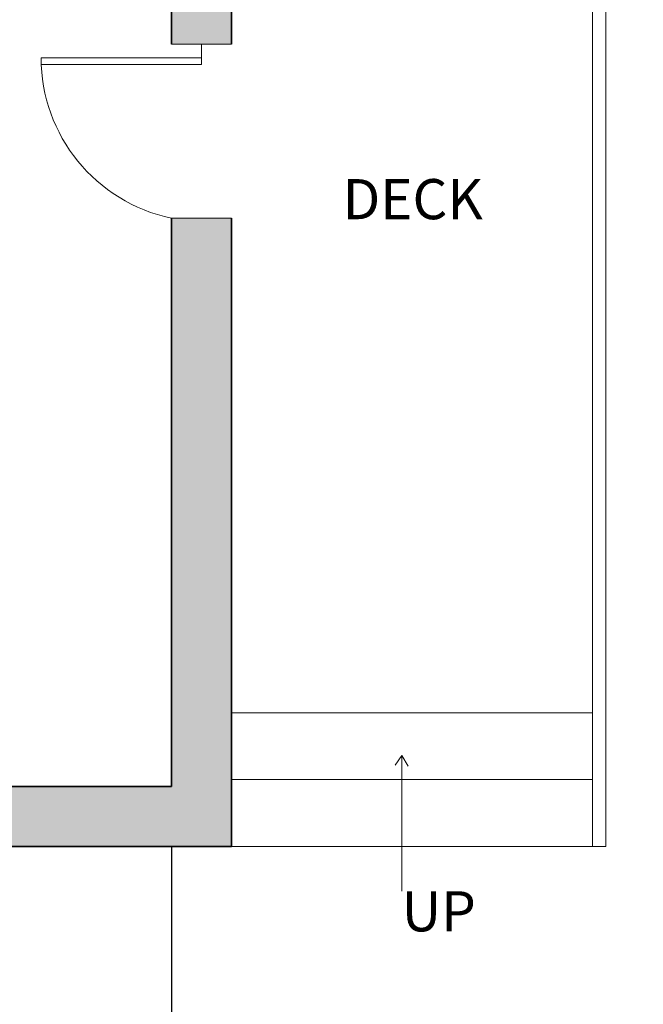
# Model space of a CAD drawing. Units: inches. Extents: x -9 to 646, y -802 to 47.
# Tile 3 of 17: x 326 to 419, y -670 to -522. Entities that reach past the tile are written whole.
import ezdxf

# ---------------------------------------------------------------- set-up
doc = ezdxf.new("R2010")
doc.units = ezdxf.units.IN
doc.header["$MEASUREMENT"] = 0
for name, color, linetype, lineweight in [('A-ANNO-SYMB', 7, 'Continuous', 13), ('A-ANNO-TEXT', 7, 'Continuous', 18), ('A-AREA-IDEN', 7, 'Continuous', 18), ('A-DOOR', 4, 'Continuous', 18), ('A-FLOR-STRS', 7, 'Continuous', 18), ('A-WALL', 7, 'Continuous', 35), ('A-WALL-PATT', 5, 'Continuous', 9), ('C-SITE', 7, 'Continuous', 25)]:
    doc.layers.add(name, color=color, linetype=linetype, lineweight=lineweight)
doc.styles.get("Standard").update_dxf_attribs({"font": 'arial.ttf'})

# ---------------------------------------------------------------- blocks, each defined once
blk = doc.blocks.new('DOOR-LEAF-24-WALL9')
for p, q in [((0, 0), (0, 24)), ((1, 0), (1, 24)), ((0, 0), (1, 0))]:
    blk.add_line(p, q)
blk.add_arc((0, -0.52), 24.52, 11.8123, 90)

msp = doc.modelspace()

# ---------------------------------------------------------------- hatches: boundary and pattern name
at = {"layer": 'A-WALL-PATT'}
h = msp.add_hatch(color=256, dxfattribs=at)
h.dxf.hatch_style = 1
h.paths.add_polyline_path([(73.4, -418.07), (63.37, -418.07), (63.37, -487.07), (63.35, -496.07), (67.87, -496.07), (67.87, -427.07), (73.4, -427.07)])
h.paths.add_polyline_path([(73.87, -487.07), (67.87, -487.07), (67.87, -496.07), (73.87, -496.07)])
h.paths.add_polyline_path([(39.37, -496.07), (39.35, -496.07), (39.35, -487.07), (30.37, -487.07), (30.37, -646.07), (69.62, -646.07), (69.62, -637.07), (39.37, -637.07)])
h.paths.add_polyline_path([(158.27, -637.07), (105.62, -637.07), (105.62, -646.07), (158.27, -646.07)])
h.paths.add_polyline_path([(286.47, -637.07), (194.27, -637.07), (194.27, -646.07), (286.47, -646.07)])
h.paths.add_polyline_path([(357.37, -552.07), (352.87, -552.07), (348.37, -552.07), (348.37, -637.07), (322.47, -637.07), (322.47, -646.07), (357.37, -646.07)])
h.paths.add_polyline_path([(357.37, -459.07), (352.87, -459.07), (348.37, -459.07), (348.37, -526.07), (357.37, -526.07), (357.37, -520.07), (363.37, -520.07), (363.37, -511.07), (357.37, -511.07)], flags=17)
h.paths.add_polyline_path([(39.37, -262.07), (213.37, -262.07), (213.37, -268.07), (222.37, -268.07), (222.37, -247.07), (213.37, -247.07), (213.37, -253.07), (39.37, -253.07), (39.37, -1.07), (222.37, -1.07), (222.37, 7.93), (30.37, 7.93), (30.37, -427.07), (39.36, -427.07), (39.36, -418.07)])
h.paths.add_polyline_path([(570.37, -149.32), (561.37, -149.32), (561.37, -161.07), (433.37, -161.07), (433.37, -165.57), (433.37, -170.07), (438.37, -170.07), (438.37, -176.07), (447.37, -176.07), (447.37, -170.07), (561.37, -170.07), (561.37, -229.57), (570.37, -229.57)])
h.paths.add_polyline_path([(570.37, -289.57), (561.37, -289.57), (561.37, -349.07), (479.37, -349.07), (479.37, -353.57), (479.37, -358.07), (561.37, -358.07), (561.37, -418.07), (447.37, -418.07), (447.37, -358.07), (453.37, -358.07), (453.37, -349.07), (447.37, -349.07), (447.37, -202.07), (442.87, -202.07), (438.37, -202.07), (438.37, -427.07), (561.37, -427.07), (561.37, -451.07), (570.37, -451.07)])
h.paths.add_polyline_path([(570.37, -496.07), (570.37, -487.07), (561.37, -487.07), (561.37, -511.07), (411.37, -511.07), (411.37, -515.57), (411.37, -520.07), (570.37, -520.07)])

# ---------------------------------------------------------------- linework, layer by layer
at = {"layer": 'A-ANNO-SYMB'}
for p, q in [((382.82, -632.47), (381.86, -633.89)), ((382.82, -652.76), (382.82, -632.47)), ((382.82, -632.47), (383.79, -634.06))]:
    msp.add_line(p, q, dxfattribs=at)
at = {"layer": 'A-DOOR'}
for p, q in [((357.37, -526.07), (348.37, -526.07)), ((352.87, -526.07), (352.87, -528.07)), ((352.87, -552.07), (348.37, -552.07)), ((352.87, -552.07), (357.37, -552.07)), ((357.37, -552.07), (357.37, -552.07))]:
    msp.add_line(p, q, dxfattribs=at)
at = {"layer": 'A-FLOR-STRS'}
for p, q in [((411.37, -520.07), (411.37, -646.07)), ((413.37, -520.07), (413.37, -646.07)), ((357.37, -626.07), (411.37, -626.07)), ((357.37, -636.07), (411.37, -636.07)), ((357.37, -646.07), (411.37, -646.07)), ((411.37, -646.07), (413.37, -646.07))]:
    msp.add_line(p, q, dxfattribs=at)
at = {"layer": 'A-WALL'}
for p, q in [((348.37, -459.07), (348.37, -526.07)), ((357.37, -520.07), (357.37, -526.07)), ((348.37, -552.07), (348.37, -637.07)), ((357.37, -552.07), (357.37, -646.07)), ((39.37, -637.07), (348.37, -637.07)), ((30.37, -646.07), (357.37, -646.07))]:
    msp.add_line(p, q, dxfattribs=at)
at = {"layer": 'C-SITE'}
msp.add_line((348.37, -646.07), (348.37, -762.07), dxfattribs=at)

# ---------------------------------------------------------------- block references
at = {"layer": 'A-DOOR', "extrusion": (0, 0, -1), "zscale": -1, "rotation": 270.0000000000002}
msp.add_blockref('DOOR-LEAF-24-WALL9', (-352.87, -528.07), dxfattribs=at)

# ---------------------------------------------------------------- texts
at = {"layer": 'A-ANNO-TEXT', "insert": (382.82, -652.76), "char_height": 6, "attachment_point": 1}
msp.add_mtext('UP', dxfattribs=at)
at = {"layer": 'A-AREA-IDEN', "insert": (373.98, -546.23), "char_height": 6, "attachment_point": 1}
msp.add_mtext('DECK', dxfattribs=at)

doc.saveas('drawing.dxf')
